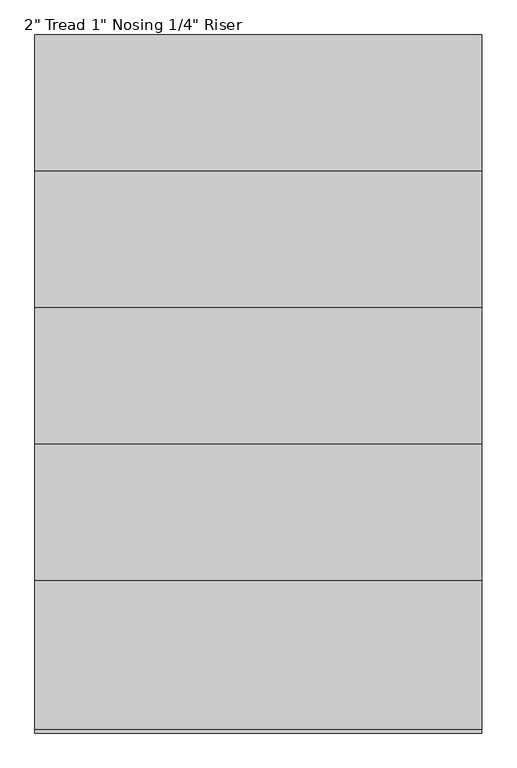
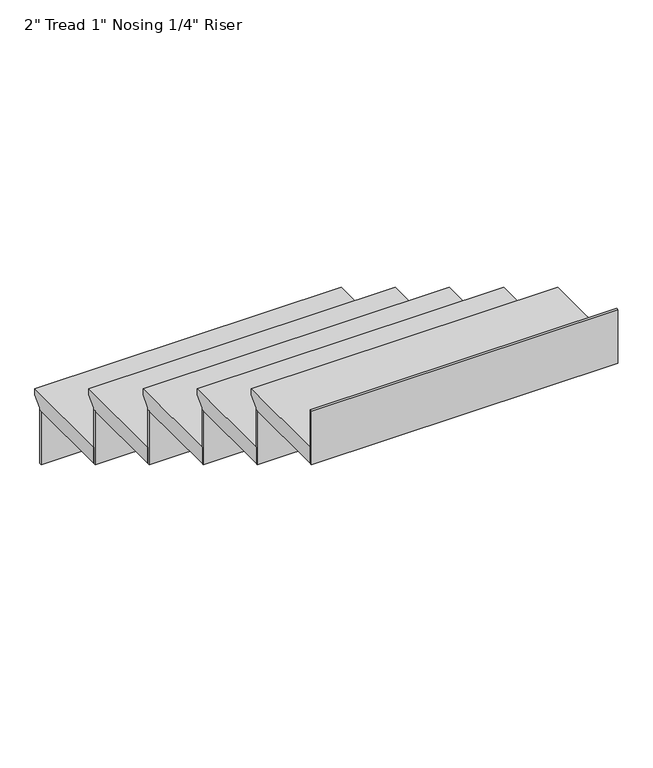
"""IFC4 building model written with IfcOpenShell, lengths in millimetres: stair flight geometry."""

from ifc_helpers import new_model, si_unit, frame, origin, place, context, project, spatial, polyline, outline, extrude, source, transform, mapped, element, save


def stair_flight_531346ed(model_context):
    return source(origin(), model_context, "Body", "SweptSolid", [
        extrude(outline(polyline([(3312.5398463, 1693.3333333), (3617.3398463, 1693.3333333), (3617.3398463, 1674.2833333), (3591.9398463, 1648.8833333), (3591.9398463, 1642.5333333), (3312.5398463, 1642.5333333), (3312.5398463, 1693.3333333)])), frame((-10599.5602428, 0.0, 0.0), z_axis=(1.0, 0.0, 0.0), x_axis=(0.0, 1.0, 0.0)), (0.0, 0.0, 1.0), 914.4),
        extrude(outline(polyline([(-10599.5602428, 3585.5898463), (-10599.5602428, 3591.9398463), (-9685.1602428, 3591.9398463), (-9685.1602428, 3585.5898463), (-10599.5602428, 3585.5898463)])), frame((0.0, 0.0, 1473.2), z_axis=(0.0, 0.0, 1.0), x_axis=(1.0, 0.0, 0.0)), (0.0, 0.0, 1.0), 169.3333333),
        extrude(outline(polyline([(-10599.5602428, 3306.1898463), (-10599.5602428, 3312.5398463), (-9685.1602428, 3312.5398463), (-9685.1602428, 3306.1898463), (-10599.5602428, 3306.1898463)])), frame((0.0, 0.0, 1642.5333333), z_axis=(0.0, 0.0, 1.0), x_axis=(1.0, 0.0, 0.0)), (0.0, 0.0, 1.0), 169.3333333),
        extrude(outline(polyline([(3033.1398463, 1862.6666667), (3337.9398463, 1862.6666667), (3337.9398463, 1843.6166667), (3312.5398463, 1818.2166667), (3312.5398463, 1811.8666667), (3033.1398463, 1811.8666667), (3033.1398463, 1862.6666667)])), frame((-10599.5602428, 0.0, 0.0), z_axis=(1.0, 0.0, 0.0), x_axis=(0.0, 1.0, 0.0)), (0.0, 0.0, 1.0), 914.4),
        extrude(outline(polyline([(-10599.5602428, 3026.7898463), (-10599.5602428, 3033.1398463), (-9685.1602428, 3033.1398463), (-9685.1602428, 3026.7898463), (-10599.5602428, 3026.7898463)])), frame((0.0, 0.0, 1811.8666667), z_axis=(0.0, 0.0, 1.0), x_axis=(1.0, 0.0, 0.0)), (0.0, 0.0, 1.0), 169.3333333),
        extrude(outline(polyline([(2753.7398463, 2032.0), (3058.5398463, 2032.0), (3058.5398463, 2012.95), (3033.1398463, 1987.55), (3033.1398463, 1981.2), (2753.7398463, 1981.2), (2753.7398463, 2032.0)])), frame((-10599.5602428, 0.0, 0.0), z_axis=(1.0, 0.0, 0.0), x_axis=(0.0, 1.0, 0.0)), (0.0, 0.0, 1.0), 914.4),
        extrude(outline(polyline([(-10599.5602428, 2747.3898463), (-10599.5602428, 2753.7398463), (-9685.1602428, 2753.7398463), (-9685.1602428, 2747.3898463), (-10599.5602428, 2747.3898463)])), frame((0.0, 0.0, 1981.2), z_axis=(0.0, 0.0, 1.0), x_axis=(1.0, 0.0, 0.0)), (0.0, 0.0, 1.0), 169.3333333),
        extrude(outline(polyline([(2474.3398463, 2201.3333333), (2779.1398463, 2201.3333333), (2779.1398463, 2182.2833333), (2753.7398463, 2156.8833333), (2753.7398463, 2150.5333333), (2474.3398463, 2150.5333333), (2474.3398463, 2201.3333333)])), frame((-10599.5602428, 0.0, 0.0), z_axis=(1.0, 0.0, 0.0), x_axis=(0.0, 1.0, 0.0)), (0.0, 0.0, 1.0), 914.4),
        extrude(outline(polyline([(-10599.5602428, 2467.9898463), (-10599.5602428, 2474.3398463), (-9685.1602428, 2474.3398463), (-9685.1602428, 2467.9898463), (-10599.5602428, 2467.9898463)])), frame((0.0, 0.0, 2150.5333333), z_axis=(0.0, 0.0, 1.0), x_axis=(1.0, 0.0, 0.0)), (0.0, 0.0, 1.0), 169.3333333),
        extrude(outline(polyline([(-10599.5602428, 2188.5898463), (-10599.5602428, 2194.9398463), (-9685.1602428, 2194.9398463), (-9685.1602428, 2188.5898463), (-10599.5602428, 2188.5898463)])), frame((0.0, 0.0, 2319.8666667), z_axis=(0.0, 0.0, 1.0), x_axis=(1.0, 0.0, 0.0)), (0.0, 0.0, 1.0), 169.3333333),
        extrude(outline(polyline([(2194.9398463, 2370.6666667), (2499.7398463, 2370.6666667), (2499.7398463, 2351.6166667), (2474.3398463, 2326.2166667), (2474.3398463, 2319.8666667), (2194.9398463, 2319.8666667), (2194.9398463, 2370.6666667)])), frame((-10599.5602428, 0.0, 0.0), z_axis=(1.0, 0.0, 0.0), x_axis=(0.0, 1.0, 0.0)), (0.0, 0.0, 1.0), 914.4),
    ])


if __name__ == "__main__":
    model = new_model("IFC4")
    model_context = context("Model", 3, world=origin())
    ifc_project = project(units=[si_unit("LENGTHUNIT", "METRE", prefix="MILLI")], contexts=[model_context])
    site = spatial("IfcSite", under=ifc_project)
    building = spatial("IfcBuilding", under=site)
    placement = place(None, origin())
    stair_flight_shape = stair_flight_531346ed(model_context)
    element("IfcStairFlight", 1, ObjectType="2\" Tread 1\" Nosing 1/4\" Riser", at=placement, inside=building, context=model_context, shape_type="MappedRepresentation", body=[
        mapped(stair_flight_shape, transform((0.0, 0.0, 0.0), x_axis=(1.0, 0.0, 0.0), y_axis=(0.0, 1.0, 0.0), z_axis=(0.0, 0.0, 1.0))),
    ])
    save(model, "model.ifc")
